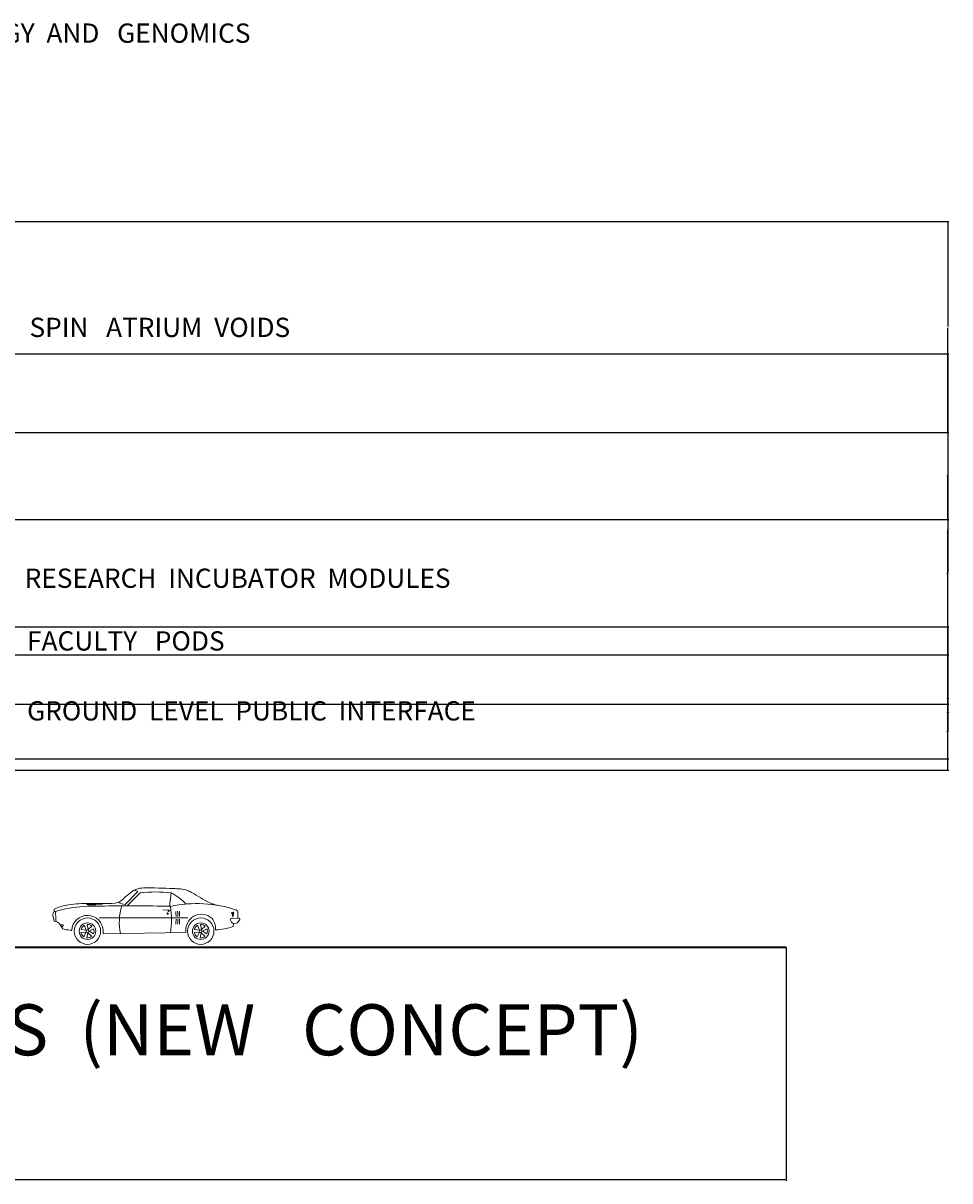
# Model space of a CAD drawing. Units: inches. Extents: x -160 to 434, y -145 to 103.
# Tile 7 of 7: x 262 to 434, y -145 to 70. Entities that reach past the tile are written whole.
import ezdxf

# ---------------------------------------------------------------- set-up
doc = ezdxf.new("R2010")
doc.units = ezdxf.units.IN
doc.header["$MEASUREMENT"] = 0
for name, color, linetype, lineweight in [('A-ANNO-DIMS', 2, 'Continuous', 18), ('A-ANNO-TEXT', 3, 'Continuous', 18), ('A-ELEV', 7, 'Continuous', 35), ('A-ENTO-VEHC', 8, 'Continuous', 13)]:
    doc.layers.add(name, color=color, linetype=linetype, lineweight=lineweight)
doc.styles.get("Standard").update_dxf_attribs({"font": 'arial.ttf'})
doc.dimstyles.get("Standard").update_dxf_attribs({"dimtxt": 0.18, "dimasz": 0.18, "dimexe": 0.18, "dimexo": 0.0625, "dimgap": 0.09, "dimtad": 0, "dimtih": 1, "dimtoh": 1, "dimdec": 4, "dimzin": 0, "dimdsep": 46, "dimtxsty": 'Standard', "dimcen": 0.09, "dimadec": 0, "dimazin": 0, "dimtfac": 1, "dimtdec": 4, "dimtofl": 0, "dimtmove": 0, "dimatfit": 3, "dimfxl": 1, "dimtolj": 1, "dimtzin": 0, "dimarcsym": 0})

# ---------------------------------------------------------------- blocks, each defined once
blk = doc.blocks.new('*U4')
for p, q in [((72.9, 40.2), (85.8, 53.2)), ((75, 38.8), (88.1, 52)), ((119.4, 51.9), (117.9, 38.3)), ((50.1, 41.1), (34.3, 41)), ((43.3, 39.8), (35.2, 39.8)), ((35.3, 40.5), (50.1, 40.6)), ((46.7, 26.8), (136.3, 26.8)), ((111.1, 34.7), (118.5, 34.6)), ((179.3, 24.4), (180.3, 22.5)), ((180.4, 26.2), (187.5, 26.4)), ((186.7, 22.2), (188.5, 24.4)), ((7.4, 19.8), (9.7, 19.8)), ((9.8, 17.9), (8.5, 17.9)), ((10.4, 19.2), (10.4, 18.6)), ((50.9, 13.5), (50.9, 10.5)), ((182.6, 21.1), (184.9, 21.3))]:
    blk.add_line(p, q)
for points in [[(35.3, 39.9), (35.3, 40.3, 0.269532), (35.1, 40.5), (34.4, 41, 0.575383), (34.2, 40.8), (34.2, 40.5, 0.269532), (34.3, 40.2), (35.1, 39.8, 0.575383)], [(31.3, 7.7), (33.5, 12.4), (28.4, 12, 0.199906)], [(28.5, 15.1), (33.6, 14.4), (31.7, 19.2, 0.199906)], [(39.2, 8.1), (35.5, 11.7), (34.2, 6.7, 0.199906)], [(34.6, 20.1), (35.6, 15), (39.5, 18.3, 0.199906)], [(41.2, 15.7), (36.7, 13.3), (41.1, 10.6, 0.199906)], [(142.8, 15.1), (148, 14.4), (146, 19.2, 0.199906)], [(145.7, 7.7), (147.9, 12.4), (142.8, 12, 0.199906)], [(153.5, 8.1), (149.8, 11.7), (148.6, 6.7, 0.199906)], [(149, 20.1), (149.9, 15), (153.9, 18.3, 0.199906)], [(155.6, 15.7), (151.1, 13.3), (155.4, 10.6, 0.199906)]]:
    blk.add_lwpolyline(points, format="xyb", close=True)
for points in [[(181.6, 27.5), (181.5, 31.9), (180.5, 32.4)], [(181.6, 27.5), (181.5, 31.9), (182.6, 32.5)], [(50.9, 10.5), (134.4, 11.8)]]:
    blk.add_lwpolyline(points)
for centre, radius in [((35, 13.3), 13.3), ((115.9, 31), 0.619), ((149.3, 13.3), 13.3), ((35, 13.3), 8.35), ((35, 13.3), 1.25), ((149.3, 13.3), 8.35), ((149.3, 13.3), 1.25)]:
    blk.add_circle(centre, radius)
for centre, radius, start, end in [((114.6, 105.1), 59.4, 237.6103, 240.9785), ((103.5, -95), 147.8, 83.8163, 95.9705), ((95.5, 3.9), 53.6, 43.2748, 63.5665), ((42.2, -111.3), 149.9, 87.8393, 105.8096), ((20.5, -3.2), 43.1, 98.5304, 116.112), ((80.1, -1364.1), 1403, 88.423, 91.3179), ((73.3, 50.5), 10.3, 230.424, 268.0085), ((118.3, 22.5), 51.2, 161.4307, 193.2363), ((145.2, -84.9), 126, 71.5283, 102.1242), ((25.7, 24.9), 94, 351.8279, 8.1674), ((79.2, 30.1), 76.3, 177.5773, 185.5205), ((35, 13.3), 15.9, 0.6373, 176.3412), ((45.6, 26.8), 78.8, 0.852, 4.6556), ((45.6, 26.8), 78.8, 355.2644, 358.8633), ((47.4, 26.9), 78.8, 0.852, 4.6556), ((47.4, 26.9), 78.8, 355.2644, 358.8633), ((49.2, 26.9), 78.8, 0.852, 4.6556), ((49.2, 26.9), 78.8, 355.2644, 358.8633), ((150.1, 14.4), 15.9, 49.2263, 189.1528), ((149.4, 16.5), 14.8, 352.7285, 41.6613), ((180.4, 24.9), 1.25, 91.939, 207.109), ((216.3, 37.8), 36.2, 188.4683, 196.5315), ((146.7, 37), 36.2, 344.7432, 352.8063), ((184.3, 32.3), 2.49, 357.932, 71.5283), ((116.6, 34.7), 70.3, 353.1942, 357.932), ((187.6, 25.2), 1.25, 320.1683, 91.939), ((9.7, 19.2), 0.623, 0.6373, 90.6373), ((9.8, 18.6), 0.623, 270.6373, 0.6373), ((162.5, 70.8), 56.2, 271.6865, 290.2774), ((182.5, 23.6), 2.49, 207.109, 273.4677), ((114.2, 37), 70.3, 344.3985, 346.9385), ((184.8, 23.8), 2.49, 273.4677, 320.1683)]:
    blk.add_arc(centre, radius, start, end)
blk.add_ellipse((116.9, 33.6), major_axis=(-0.63, -0.007), ratio=0.610043)
for points, knots in [([(11.4, 38.9), (18.1, 40.2), (30.9, 42), (64.8, 40.1), (70.2, 44.9), (82.4, 56.4), (99.2, 57.3), (116.1, 56.4), (133, 55.9), (145.2, 49.9), (153.6, 43.8), (161.2, 40.7), (164.9, 39.7), (167.3, 39.2)], [18.629823, 18.629823, 18.629823, 18.629823, 19.527405, 20.700571, 21.107983, 21.608568, 21.92336, 23.151359, 23.716171, 23.908743, 24.77794, 24.943072, 25.187755, 25.187755, 25.187755, 25.187755]), ([(19.1, 14.4), (19, 14.2), (18.5, 13.8), (15.4, 15), (9.2, 13.9), (7.3, 22.2), (3, 22.7), (1.3, 23.6), (0.6, 26.9), (-1, 31.5), (1.5, 32.6), (1.5, 34.1), (1.5, 34.8), (1.5, 35.1), (1.5, 35.3), (1.6, 35.5)], [16.815853, 16.815853, 16.815853, 16.815853, 16.838212, 16.885395, 17.18439, 17.479846, 17.654423, 17.670693, 17.696923, 18.016358, 18.052739, 18.140805, 18.140805, 18.140805, 18.172382, 18.172382, 18.172382, 18.172382])]:
    blk.add_open_spline(points, degree=3, knots=knots)
blk = doc.blocks.new('*D12')
at = {"layer": 'A-ANNO-DIMS', "color": 0, "lineweight": -2, "transparency": 16777216}
for p, q in [((-84.07, -101.41), (-84.07, -144.81)), ((403.75, -101.41), (403.75, -144.81)), ((-83.89, -144.63), (159.44, -144.63)), ((403.57, -144.63), (160.24, -144.63))]:
    blk.add_line(p, q, dxfattribs=at)
at = {"layer": 'A-ANNO-DIMS', "color": 0, "transparency": 16777216}
for points in [[(-83.89, -144.6), (-83.89, -144.66), (-84.07, -144.63)], [(403.57, -144.6), (403.57, -144.66), (403.75, -144.63)]]:
    blk.add_solid(points, dxfattribs=at)
at = {"layer": 'Defpoints', "color": 0, "transparency": 16777216}
for p in [(-84.07, -101.35), (403.75, -101.35), (403.75, -144.63)]:
    blk.add_point(p, dxfattribs=at)
at = {"layer": 'A-ANNO-DIMS', "color": 0, "transparency": 16777216, "insert": (159.84, -144.63), "char_height": 0.18, "attachment_point": 5}
blk.add_mtext('\\A1;487.8', dxfattribs=at)
blk = doc.blocks.new('*D31')
at = {"layer": 'A-ANNO-DIMS', "color": 0, "lineweight": -2, "transparency": 16777216}
for p, q in [((107.33, 8.95), (433.98, 8.95)), ((433.8, 8.77), (433.8, -23.43)), ((433.8, -55.99), (433.8, -23.79)), ((107.33, -56.17), (433.98, -56.17))]:
    blk.add_line(p, q, dxfattribs=at)
at = {"layer": 'A-ANNO-DIMS', "color": 0, "transparency": 16777216}
for points in [[(433.77, 8.77), (433.83, 8.77), (433.8, 8.95)], [(433.77, -55.99), (433.83, -55.99), (433.8, -56.17)]]:
    blk.add_solid(points, dxfattribs=at)
at = {"layer": 'Defpoints', "color": 0, "transparency": 16777216}
for p in [(107.27, 8.95), (107.27, -56.17), (433.8, -56.17)]:
    blk.add_point(p, dxfattribs=at)
at = {"layer": 'A-ANNO-DIMS', "color": 0, "transparency": 16777216, "insert": (433.8, -23.61), "char_height": 0.18, "attachment_point": 5}
blk.add_mtext('\\A1;65.11', dxfattribs=at)
blk = doc.blocks.new('*D32')
at = {"layer": 'A-ANNO-DIMS', "color": 0, "lineweight": -2, "transparency": 16777216}
for p, q in [((107.33, -56.17), (433.98, -56.17)), ((433.8, -56.35), (433.8, -61.07)), ((433.8, -66.15), (433.8, -61.43)), ((106.73, -66.33), (433.98, -66.33))]:
    blk.add_line(p, q, dxfattribs=at)
at = {"layer": 'A-ANNO-DIMS', "color": 0, "transparency": 16777216}
for points in [[(433.77, -56.35), (433.83, -56.35), (433.8, -56.17)], [(433.77, -66.15), (433.83, -66.15), (433.8, -66.33)]]:
    blk.add_solid(points, dxfattribs=at)
at = {"layer": 'Defpoints', "color": 0, "transparency": 16777216}
for p in [(107.27, -56.17), (106.67, -66.33), (433.8, -66.33)]:
    blk.add_point(p, dxfattribs=at)
at = {"layer": 'A-ANNO-DIMS', "color": 0, "transparency": 16777216, "insert": (433.8, -61.25), "char_height": 0.18, "attachment_point": 5}
blk.add_mtext('\\A1;10.165', dxfattribs=at)
blk = doc.blocks.new('*D40')
at = {"layer": 'A-ANNO-DIMS', "color": 0, "lineweight": -2, "transparency": 16777216}
for p, q in [((219.11, 33.57), (433.98, 33.57)), ((433.8, 33.39), (433.8, 14.15)), ((433.8, -5.46), (433.8, 13.79)), ((218.99, -5.64), (433.98, -5.64))]:
    blk.add_line(p, q, dxfattribs=at)
at = {"layer": 'A-ANNO-DIMS', "color": 0, "transparency": 16777216}
for points in [[(433.77, 33.39), (433.83, 33.39), (433.8, 33.57)], [(433.77, -5.46), (433.83, -5.46), (433.8, -5.64)]]:
    blk.add_solid(points, dxfattribs=at)
at = {"layer": 'Defpoints', "color": 0, "transparency": 16777216}
for p in [(219.05, 33.57), (218.92, -5.64), (433.8, -5.64)]:
    blk.add_point(p, dxfattribs=at)
at = {"layer": 'A-ANNO-DIMS', "color": 0, "transparency": 16777216, "insert": (433.8, 13.97), "char_height": 0.18, "attachment_point": 5}
blk.add_mtext('\\A1;39.206', dxfattribs=at)
blk = doc.blocks.new('*D42')
at = {"layer": 'A-ANNO-DIMS', "color": 0, "lineweight": -2, "transparency": 16777216}
for p, q in [((222.59, -21.84), (433.98, -21.84)), ((433.8, -22.02), (433.8, -31.63)), ((433.8, -41.61), (433.8, -31.99)), ((222.62, -41.79), (433.98, -41.79))]:
    blk.add_line(p, q, dxfattribs=at)
at = {"layer": 'A-ANNO-DIMS', "color": 0, "transparency": 16777216}
for points in [[(433.77, -22.02), (433.83, -22.02), (433.8, -21.84)], [(433.77, -41.61), (433.83, -41.61), (433.8, -41.79)]]:
    blk.add_solid(points, dxfattribs=at)
at = {"layer": 'Defpoints', "color": 0, "transparency": 16777216}
for p in [(222.53, -21.84), (222.55, -41.79), (433.8, -41.79)]:
    blk.add_point(p, dxfattribs=at)
at = {"layer": 'A-ANNO-DIMS', "color": 0, "transparency": 16777216, "insert": (433.8, -31.81), "char_height": 0.18, "attachment_point": 5}
blk.add_mtext('\\A1;19.946', dxfattribs=at)
blk = doc.blocks.new('*D43')
at = {"layer": 'A-ANNO-DIMS', "color": 0, "lineweight": -2, "transparency": 16777216}
for p, q in [((222.5, -5.64), (433.98, -5.64)), ((433.8, -5.82), (433.8, -13.56)), ((433.8, -21.66), (433.8, -13.92)), ((222.59, -21.84), (433.98, -21.84))]:
    blk.add_line(p, q, dxfattribs=at)
at = {"layer": 'A-ANNO-DIMS', "color": 0, "transparency": 16777216}
for points in [[(433.77, -5.82), (433.83, -5.82), (433.8, -5.64)], [(433.77, -21.66), (433.83, -21.66), (433.8, -21.84)]]:
    blk.add_solid(points, dxfattribs=at)
at = {"layer": 'Defpoints', "color": 0, "transparency": 16777216}
for p in [(222.44, -5.64), (222.53, -21.84), (433.8, -21.84)]:
    blk.add_point(p, dxfattribs=at)
at = {"layer": 'A-ANNO-DIMS', "color": 0, "transparency": 16777216, "insert": (433.8, -13.74), "char_height": 0.18, "attachment_point": 5}
blk.add_mtext('\\A1;16.204', dxfattribs=at)
blk = doc.blocks.new('*D45')
at = {"layer": 'A-ANNO-DIMS', "color": 0, "lineweight": -2, "transparency": 16777216}
for p, q in [((228.31, -47.01), (433.98, -47.01)), ((433.8, -47.19), (433.8, -57.57)), ((433.8, -68.3), (433.8, -57.93)), ((228.35, -68.48), (433.98, -68.48))]:
    blk.add_line(p, q, dxfattribs=at)
at = {"layer": 'A-ANNO-DIMS', "color": 0, "transparency": 16777216}
for points in [[(433.77, -47.19), (433.83, -47.19), (433.8, -47.01)], [(433.77, -68.3), (433.83, -68.3), (433.8, -68.48)]]:
    blk.add_solid(points, dxfattribs=at)
at = {"layer": 'Defpoints', "color": 0, "transparency": 16777216}
for p in [(228.25, -47.01), (228.29, -68.48), (433.8, -68.48)]:
    blk.add_point(p, dxfattribs=at)
at = {"layer": 'A-ANNO-DIMS', "color": 0, "transparency": 16777216, "insert": (433.8, -57.75), "char_height": 0.18, "attachment_point": 5}
blk.add_mtext('\\A1;21.473', dxfattribs=at)
blk = doc.blocks.new('*D46')
at = {"layer": 'A-ANNO-DIMS', "color": 0, "lineweight": -2, "transparency": 16777216}
for p, q in [((222.62, -41.79), (433.98, -41.79)), ((433.8, -41.97), (433.8, -54.95)), ((433.8, -68.3), (433.8, -55.32)), ((228.35, -68.48), (433.98, -68.48))]:
    blk.add_line(p, q, dxfattribs=at)
at = {"layer": 'A-ANNO-DIMS', "color": 0, "transparency": 16777216}
for points in [[(433.77, -41.97), (433.83, -41.97), (433.8, -41.79)], [(433.77, -68.3), (433.83, -68.3), (433.8, -68.48)]]:
    blk.add_solid(points, dxfattribs=at)
at = {"layer": 'Defpoints', "color": 0, "transparency": 16777216}
for p in [(222.55, -41.79), (228.29, -68.48), (433.8, -68.48)]:
    blk.add_point(p, dxfattribs=at)
at = {"layer": 'A-ANNO-DIMS', "color": 0, "transparency": 16777216, "insert": (433.8, -55.14), "char_height": 0.18, "attachment_point": 5}
blk.add_mtext('\\A1;26.7', dxfattribs=at)

msp = doc.modelspace()

# ---------------------------------------------------------------- linework, layer by layer
at = {"layer": 'A-ELEV'}
msp.add_line((2.6577, -101.346), (403.7477, -101.346), dxfattribs=at)

# ---------------------------------------------------------------- block references
at = {"layer": 'A-ENTO-VEHC', "xscale": 0.1843091790693797, "yscale": 0.1843091790693797, "zscale": 0.1843091790693797}
msp.add_blockref('*U4', (267.3481, -100.8377), dxfattribs=at)

# ---------------------------------------------------------------- texts
at = {"layer": 'A-ANNO-TEXT'}
for s, height, p in [('POD  B :  BIOTECHNOLOGY  AND   GENOMICS', 3.579169, (203.7515, 66.798)), ('SPIN   ATRIUM  VOIDS', 3.579169, (263.0185, 12.0865)), ('RESEARCH  INCUBATOR  MODULES  ', 3.579169, (262.1205, -34.5527)), ('FACULTY   PODS', 3.579169, (262.5695, -46.2126)), ('GROUND  LEVEL  PUBLIC  INTERFACE  ', 3.579169, (262.5695, -59.2177)), ('FRONT   ELEVATION - RESEARCH   SPINE   AND  COLLABORATION   PODS  (NEW   CONCEPT)', 9.480943, (-160.9184, -121.4719))]:
    msp.add_text(s, height=height, dxfattribs=at).set_placement(p)

# ---------------------------------------------------------------- dimensions: what is measured, and where the dimension line sits
at = {"layer": 'A-ANNO-DIMS'}
for base, p1, p2, override, picture, middle in [((433.7977, -5.6358), (219.0478, 33.5699), (218.9244, -5.6358), {"dimdec": 3, "dimlfac": 1, "dimrnd": 0, "dimzin": 0, "dimdsep": 46, "dimlunit": 2}, '*D40', (433.7977, 13.9671)), ((433.7977, -56.1669), (107.2684, 8.9457), (107.2684, -56.1669), {"dimdec": 2, "dimlfac": 1, "dimrnd": 0, "dimzin": 0, "dimdsep": 46, "dimlunit": 2}, '*D31', (433.7977, -23.6106)), ((433.7977, -21.8399), (222.4353, -5.6358), (222.5284, -21.8399), {"dimdec": 3, "dimlfac": 1, "dimrnd": 0, "dimzin": 0, "dimdsep": 46, "dimlunit": 2}, '*D43', (433.7977, -13.7378)), ((433.7977, -41.7856), (222.5284, -21.8399), (222.553, -41.7856), {"dimdec": 3, "dimlfac": 1, "dimrnd": 0, "dimzin": 0, "dimdsep": 46, "dimlunit": 2}, '*D42', (433.7977, -31.8128)), ((433.7977, -68.4846), (222.553, -41.7856), (228.2854, -68.4846), {"dimdec": 1, "dimlfac": 1, "dimrnd": 0, "dimzin": 0, "dimdsep": 46, "dimlunit": 2}, '*D46', (433.7977, -55.1351)), ((433.79775, -68.48461), (228.24902, -47.01209), (228.28543, -68.48461), {"dimdec": 3, "dimlfac": 1, "dimrnd": 0, "dimzin": 0, "dimdsep": 46, "dimlunit": 2}, '*D45', (433.79775, -57.74835)), ((433.7977, -66.3322), (107.2684, -56.1669), (106.6672, -66.3322), {"dimdec": 3, "dimlfac": 1, "dimrnd": 0, "dimzin": 0, "dimdsep": 46, "dimlunit": 2}, '*D32', (433.7977, -61.2496))]:
    dim = msp.add_linear_dim(base=base, p1=p1, p2=p2, angle=90, dimstyle='Standard', override=override, dxfattribs=at)
    dim.commit()
    dim.dimension.update_dxf_attribs({"geometry": picture, "text_midpoint": middle})
dim = msp.add_linear_dim(base=(403.7477, -144.6322), p1=(-84.0722, -101.346), p2=(403.7477, -101.346), dimstyle='Standard', override={"dimdec": 1, "dimlfac": 1, "dimrnd": 0, "dimzin": 0, "dimdsep": 46, "dimlunit": 2}, dxfattribs=at)
dim.commit()
dim.dimension.update_dxf_attribs({"geometry": '*D12', "text_midpoint": (159.8378, -144.6322)})

doc.saveas('drawing.dxf')
